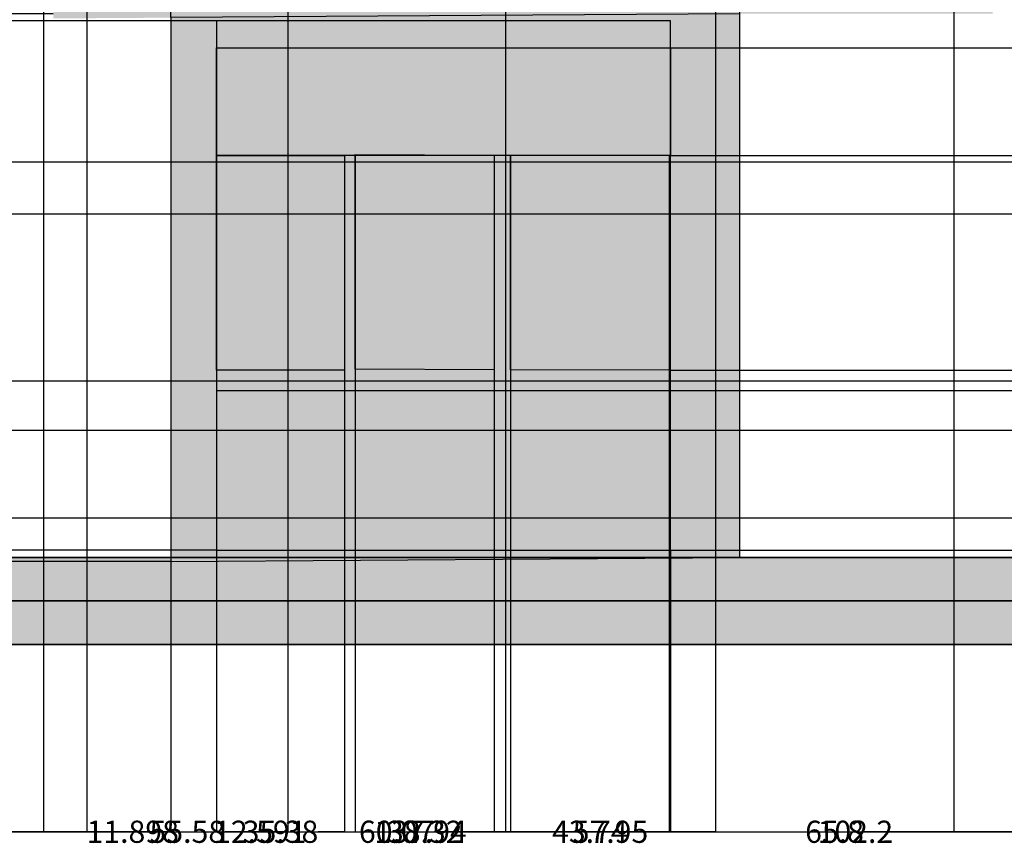
# Model space of a CAD drawing. Units: inches. Extents: x -655 to 499, y 20 to 616.
# Tile 2 of 7: x -409 to -137, y 20 to 248. Entities that reach past the tile are written whole.
import ezdxf

# ---------------------------------------------------------------- set-up
doc = ezdxf.new("R2010")
doc.units = ezdxf.units.IN
doc.header["$MEASUREMENT"] = 0
for name, color, linetype, lineweight in [('A-ANNO-DIMS', 2, 'Continuous', 18), ('A-ELEV', 7, 'Continuous', 35), ('A-ELEV-PATT', 9, 'Continuous', 13), ('A-GLAZ', 3, 'Continuous', 25), ('C-TOPO', 18, 'Continuous', 18)]:
    doc.layers.add(name, color=color, linetype=linetype, lineweight=lineweight)
doc.styles.get("Standard").update_dxf_attribs({"font": 'arial.ttf'})
doc.dimstyles.get("Standard").update_dxf_attribs({"dimtxt": 6.125, "dimasz": 0.18, "dimexe": 0.18, "dimexo": 0.0625, "dimgap": 0.09, "dimtad": 0, "dimtih": 1, "dimtoh": 1, "dimdec": 4, "dimzin": 0, "dimdsep": 46, "dimlunit": 4, "dimtxsty": 'Standard', "dimcen": 0.09, "dimadec": 0, "dimazin": 0, "dimtfac": 1, "dimtdec": 4, "dimtofl": 0, "dimtmove": 0, "dimatfit": 3, "dimfxl": 1, "dimtolj": 1, "dimtzin": 0, "dimarcsym": 0})

# ---------------------------------------------------------------- blocks, each defined once
blk = doc.blocks.new('*D10')
at = {"layer": 'A-ANNO-DIMS', "color": 0, "lineweight": -2, "transparency": 16777216}
for p, q in [((434.11, 393.11), (434.11, 23.7)), ((-590.16, 75.57), (-590.16, 23.7)), ((-589.98, 23.88), (-90.54, 23.88)), ((433.93, 23.88), (-65.51, 23.88))]:
    blk.add_line(p, q, dxfattribs=at)
at = {"layer": 'A-ANNO-DIMS', "color": 0, "transparency": 16777216}
for points in [[(-589.98, 23.91), (-589.98, 23.85), (-590.16, 23.88)], [(433.93, 23.91), (433.93, 23.85), (434.11, 23.88)]]:
    blk.add_solid(points, dxfattribs=at)
at = {"layer": 'Defpoints', "color": 0, "transparency": 16777216}
for p in [(434.11, 393.17), (-590.16, 75.63), (434.11, 23.88)]:
    blk.add_point(p, dxfattribs=at)
at = {"layer": 'A-ANNO-DIMS', "color": 0, "transparency": 16777216, "insert": (-78.02, 23.88), "char_height": 6.125, "attachment_point": 5}
blk.add_mtext('\\A1;1024.3', dxfattribs=at)
blk = doc.blocks.new('*D12')
at = {"layer": 'A-ANNO-DIMS', "color": 0, "lineweight": -2, "transparency": 16777216}
for p, q in [((-493.03, 99.57), (-493.03, 23.7)), ((-366.94, 98.47), (-366.94, 23.7)), ((-492.85, 23.88), (-439.53, 23.88)), ((-367.12, 23.88), (-420.44, 23.88))]:
    blk.add_line(p, q, dxfattribs=at)
at = {"layer": 'A-ANNO-DIMS', "color": 0, "transparency": 16777216}
for points in [[(-492.85, 23.91), (-492.85, 23.85), (-493.03, 23.88)], [(-367.12, 23.91), (-367.12, 23.85), (-366.94, 23.88)]]:
    blk.add_solid(points, dxfattribs=at)
at = {"layer": 'Defpoints', "color": 0, "transparency": 16777216}
for p in [(-493.03, 99.63), (-366.94, 98.53), (-366.94, 23.88)]:
    blk.add_point(p, dxfattribs=at)
at = {"layer": 'A-ANNO-DIMS', "color": 0, "transparency": 16777216, "insert": (-429.99, 23.88), "char_height": 6.125, "attachment_point": 5}
blk.add_mtext('\\A1;126.1', dxfattribs=at)
blk = doc.blocks.new('*D13')
at = {"layer": 'A-ANNO-DIMS', "color": 0, "lineweight": -2, "transparency": 16777216}
for p, q in [((-229.01, 101.57), (-229.01, 23.7)), ((-366.94, 98.47), (-366.94, 23.7)), ((-366.76, 23.88), (-310.48, 23.88)), ((-229.19, 23.88), (-285.47, 23.88))]:
    blk.add_line(p, q, dxfattribs=at)
at = {"layer": 'A-ANNO-DIMS', "color": 0, "transparency": 16777216}
for points in [[(-366.76, 23.91), (-366.76, 23.85), (-366.94, 23.88)], [(-229.19, 23.91), (-229.19, 23.85), (-229.01, 23.88)]]:
    blk.add_solid(points, dxfattribs=at)
at = {"layer": 'Defpoints', "color": 0, "transparency": 16777216}
for p in [(-229.01, 101.63), (-366.94, 98.53), (-229.01, 23.88)]:
    blk.add_point(p, dxfattribs=at)
at = {"layer": 'A-ANNO-DIMS', "color": 0, "transparency": 16777216, "insert": (-297.98, 23.88), "char_height": 6.125, "attachment_point": 5}
blk.add_mtext('\\A1;137.94', dxfattribs=at)
blk = doc.blocks.new('*D14')
at = {"layer": 'A-ANNO-DIMS', "color": 0, "lineweight": -2, "transparency": 16777216}
for p, q in [((-229.01, 101.57), (-229.01, 23.7)), ((-126.81, 99.57), (-126.81, 23.7)), ((-228.83, 23.88), (-188.01, 23.88)), ((-126.99, 23.88), (-167.8, 23.88))]:
    blk.add_line(p, q, dxfattribs=at)
at = {"layer": 'A-ANNO-DIMS', "color": 0, "transparency": 16777216}
for points in [[(-228.83, 23.91), (-228.83, 23.85), (-229.01, 23.88)], [(-126.99, 23.91), (-126.99, 23.85), (-126.81, 23.88)]]:
    blk.add_solid(points, dxfattribs=at)
at = {"layer": 'Defpoints', "color": 0, "transparency": 16777216}
for p in [(-229.01, 101.63), (-126.81, 99.63), (-126.81, 23.88)]:
    blk.add_point(p, dxfattribs=at)
at = {"layer": 'A-ANNO-DIMS', "color": 0, "transparency": 16777216, "insert": (-177.91, 23.88), "char_height": 6.125, "attachment_point": 5}
blk.add_mtext('\\A1;102.2', dxfattribs=at)
blk = doc.blocks.new('*D21')
at = {"layer": 'A-ANNO-DIMS', "color": 0, "lineweight": -2, "transparency": 16777216}
for p, q in [((179.11, 559.78), (486.04, 559.78)), ((485.86, 559.6), (485.86, 320.92)), ((485.86, 75.81), (485.86, 314.49)), ((-590.1, 75.63), (486.04, 75.63))]:
    blk.add_line(p, q, dxfattribs=at)
at = {"layer": 'A-ANNO-DIMS', "color": 0, "transparency": 16777216}
for points in [[(485.83, 559.6), (485.89, 559.6), (485.86, 559.78)], [(485.83, 75.81), (485.89, 75.81), (485.86, 75.63)]]:
    blk.add_solid(points, dxfattribs=at)
at = {"layer": 'Defpoints', "color": 0, "transparency": 16777216}
for p in [(179.05, 559.78), (485.86, 559.78), (-590.16, 75.63)]:
    blk.add_point(p, dxfattribs=at)
at = {"layer": 'A-ANNO-DIMS', "color": 0, "transparency": 16777216, "insert": (485.86, 317.7), "char_height": 6.125, "attachment_point": 5}
blk.add_mtext('\\A1;484.15', dxfattribs=at)
blk = doc.blocks.new('*D25')
at = {"layer": 'A-ANNO-DIMS', "color": 0, "lineweight": -2, "transparency": 16777216}
for p, q in [((-399.44, 249.84), (-642.09, 249.84)), ((-641.91, 249.66), (-641.91, 177.41)), ((-641.91, 98.71), (-641.91, 170.97)), ((-367.01, 98.53), (-642.09, 98.53))]:
    blk.add_line(p, q, dxfattribs=at)
at = {"layer": 'A-ANNO-DIMS', "color": 0, "transparency": 16777216}
for points in [[(-641.94, 249.66), (-641.88, 249.66), (-641.91, 249.84)], [(-641.94, 98.71), (-641.88, 98.71), (-641.91, 98.53)]]:
    blk.add_solid(points, dxfattribs=at)
at = {"layer": 'Defpoints', "color": 0, "transparency": 16777216}
for p in [(-399.38, 249.84), (-641.91, 98.53), (-366.94, 98.53)]:
    blk.add_point(p, dxfattribs=at)
at = {"layer": 'A-ANNO-DIMS', "color": 0, "transparency": 16777216, "insert": (-641.91, 174.19), "char_height": 6.125, "attachment_point": 5}
blk.add_mtext('\\A1;151.3', dxfattribs=at)
blk = doc.blocks.new('*D38')
at = {"layer": 'A-ANNO-DIMS', "color": 0, "lineweight": -2, "transparency": 16777216}
for p, q in [((-402.07, 316.99), (-402.07, 23.7)), ((-390.18, 316.99), (-390.18, 23.7)), ((-401.89, 23.88), (-390.36, 23.88)), ((-390.18, 23.88), (-390, 23.88))]:
    blk.add_line(p, q, dxfattribs=at)
at = {"layer": 'A-ANNO-DIMS', "color": 0, "transparency": 16777216}
for points in [[(-401.89, 23.91), (-401.89, 23.85), (-402.07, 23.88)], [(-390.36, 23.91), (-390.36, 23.85), (-390.18, 23.88)]]:
    blk.add_solid(points, dxfattribs=at)
at = {"layer": 'Defpoints', "color": 0, "transparency": 16777216}
for p in [(-402.07, 317.05), (-390.18, 317.05), (-390.18, 23.88)]:
    blk.add_point(p, dxfattribs=at)
at = {"layer": 'A-ANNO-DIMS', "color": 0, "transparency": 16777216, "insert": (-377.47, 23.88), "char_height": 6.125, "attachment_point": 5}
blk.add_mtext('\\A1;11.898', dxfattribs=at)
blk = doc.blocks.new('*D39')
at = {"layer": 'A-ANNO-DIMS', "color": 0, "lineweight": -2, "transparency": 16777216}
for p, q in [((-390.18, 316.99), (-390.18, 23.7)), ((-334.6, 316.99), (-334.6, 23.7)), ((-390, 23.88), (-372.82, 23.88)), ((-334.78, 23.88), (-351.96, 23.88))]:
    blk.add_line(p, q, dxfattribs=at)
at = {"layer": 'A-ANNO-DIMS', "color": 0, "transparency": 16777216}
for points in [[(-390, 23.91), (-390, 23.85), (-390.18, 23.88)], [(-334.78, 23.91), (-334.78, 23.85), (-334.6, 23.88)]]:
    blk.add_solid(points, dxfattribs=at)
at = {"layer": 'Defpoints', "color": 0, "transparency": 16777216}
for p in [(-390.18, 317.05), (-334.6, 317.05), (-334.6, 23.88)]:
    blk.add_point(p, dxfattribs=at)
at = {"layer": 'A-ANNO-DIMS', "color": 0, "transparency": 16777216, "insert": (-362.39, 23.88), "char_height": 6.125, "attachment_point": 5}
blk.add_mtext('\\A1;55.58', dxfattribs=at)
blk = doc.blocks.new('*D40')
at = {"layer": 'A-ANNO-DIMS', "color": 0, "lineweight": -2, "transparency": 16777216}
for p, q in [((-334.6, 316.99), (-334.6, 23.7)), ((-274.52, 316.99), (-274.52, 23.7)), ((-334.42, 23.88), (-315, 23.88)), ((-274.7, 23.88), (-294.12, 23.88))]:
    blk.add_line(p, q, dxfattribs=at)
at = {"layer": 'A-ANNO-DIMS', "color": 0, "transparency": 16777216}
for points in [[(-334.42, 23.91), (-334.42, 23.85), (-334.6, 23.88)], [(-274.7, 23.91), (-274.7, 23.85), (-274.52, 23.88)]]:
    blk.add_solid(points, dxfattribs=at)
at = {"layer": 'Defpoints', "color": 0, "transparency": 16777216}
for p in [(-334.6, 317.05), (-274.52, 317.05), (-274.52, 23.88)]:
    blk.add_point(p, dxfattribs=at)
at = {"layer": 'A-ANNO-DIMS', "color": 0, "transparency": 16777216, "insert": (-304.56, 23.88), "char_height": 6.125, "attachment_point": 5}
blk.add_mtext('\\A1;60.07', dxfattribs=at)
blk = doc.blocks.new('*D41')
at = {"layer": 'A-ANNO-DIMS', "color": 0, "lineweight": -2, "transparency": 16777216}
for p, q in [((-274.52, 316.99), (-274.52, 23.7)), ((-216.57, 316.99), (-216.57, 23.7)), ((-274.34, 23.88), (-256, 23.88)), ((-216.75, 23.88), (-235.1, 23.88))]:
    blk.add_line(p, q, dxfattribs=at)
at = {"layer": 'A-ANNO-DIMS', "color": 0, "transparency": 16777216}
for points in [[(-274.34, 23.91), (-274.34, 23.85), (-274.52, 23.88)], [(-216.75, 23.91), (-216.75, 23.85), (-216.57, 23.88)]]:
    blk.add_solid(points, dxfattribs=at)
at = {"layer": 'Defpoints', "color": 0, "transparency": 16777216}
for p in [(-274.52, 317.05), (-216.57, 317.05), (-216.57, 23.88)]:
    blk.add_point(p, dxfattribs=at)
at = {"layer": 'A-ANNO-DIMS', "color": 0, "transparency": 16777216, "insert": (-245.55, 23.88), "char_height": 6.125, "attachment_point": 5}
blk.add_mtext('\\A1;57.95', dxfattribs=at)
blk = doc.blocks.new('*D42')
at = {"layer": 'A-ANNO-DIMS', "color": 0, "lineweight": -2, "transparency": 16777216}
for p, q in [((-216.57, 316.99), (-216.57, 23.7)), ((-150.77, 316.99), (-150.77, 23.7)), ((-216.39, 23.88), (-191.74, 23.88)), ((-150.95, 23.88), (-175.6, 23.88))]:
    blk.add_line(p, q, dxfattribs=at)
at = {"layer": 'A-ANNO-DIMS', "color": 0, "transparency": 16777216}
for points in [[(-216.39, 23.91), (-216.39, 23.85), (-216.57, 23.88)], [(-150.95, 23.91), (-150.95, 23.85), (-150.77, 23.88)]]:
    blk.add_solid(points, dxfattribs=at)
at = {"layer": 'Defpoints', "color": 0, "transparency": 16777216}
for p in [(-216.57, 317.05), (-150.77, 317.05), (-150.77, 23.88)]:
    blk.add_point(p, dxfattribs=at)
at = {"layer": 'A-ANNO-DIMS', "color": 0, "transparency": 16777216, "insert": (-183.67, 23.88), "char_height": 6.125, "attachment_point": 5}
blk.add_mtext('\\A1;65.8', dxfattribs=at)
blk = doc.blocks.new('*D43')
at = {"layer": 'A-ANNO-DIMS', "color": 0, "lineweight": -2, "transparency": 16777216}
for p, q in [((-366.94, 248.81), (-366.94, 611.71)), ((-366.76, 611.53), (-300.88, 611.53)), ((-209.98, 611.53), (-275.87, 611.53)), ((-209.8, 99.69), (-209.8, 611.71))]:
    blk.add_line(p, q, dxfattribs=at)
at = {"layer": 'A-ANNO-DIMS', "color": 0, "transparency": 16777216}
for points in [[(-366.76, 611.56), (-366.76, 611.5), (-366.94, 611.53)], [(-209.98, 611.56), (-209.98, 611.5), (-209.8, 611.53)]]:
    blk.add_solid(points, dxfattribs=at)
at = {"layer": 'Defpoints', "color": 0, "transparency": 16777216}
for p in [(-209.8, 611.53), (-366.94, 248.74), (-209.8, 99.63)]:
    blk.add_point(p, dxfattribs=at)
at = {"layer": 'A-ANNO-DIMS', "color": 0, "transparency": 16777216, "insert": (-288.37, 611.53), "char_height": 6.125, "attachment_point": 5}
blk.add_mtext('\\A1;157.14', dxfattribs=at)
blk = doc.blocks.new('*D44')
at = {"layer": 'A-ANNO-DIMS', "color": 0, "lineweight": -2, "transparency": 16777216}
for p, q in [((-366.94, 248.68), (-366.94, 23.7)), ((-354.35, 247.78), (-354.35, 23.7)), ((-366.76, 23.88), (-354.53, 23.88)), ((-354.35, 23.88), (-354.17, 23.88))]:
    blk.add_line(p, q, dxfattribs=at)
at = {"layer": 'A-ANNO-DIMS', "color": 0, "transparency": 16777216}
for points in [[(-366.76, 23.91), (-366.76, 23.85), (-366.94, 23.88)], [(-354.53, 23.91), (-354.53, 23.85), (-354.35, 23.88)]]:
    blk.add_solid(points, dxfattribs=at)
at = {"layer": 'Defpoints', "color": 0, "transparency": 16777216}
for p in [(-366.94, 248.74), (-354.35, 247.84), (-354.35, 23.88)]:
    blk.add_point(p, dxfattribs=at)
at = {"layer": 'A-ANNO-DIMS', "color": 0, "transparency": 16777216, "insert": (-342.25, 23.88), "char_height": 6.125, "attachment_point": 5}
blk.add_mtext('\\A1;12.591', dxfattribs=at)
blk = doc.blocks.new('*D45')
at = {"layer": 'A-ANNO-DIMS', "color": 0, "lineweight": -2, "transparency": 16777216}
for p, q in [((-354.35, 210.58), (-354.35, 23.7)), ((-318.97, 210.58), (-318.97, 23.7)), ((-354.17, 23.88), (-347.09, 23.88)), ((-319.15, 23.88), (-326.24, 23.88))]:
    blk.add_line(p, q, dxfattribs=at)
at = {"layer": 'A-ANNO-DIMS', "color": 0, "transparency": 16777216}
for points in [[(-354.17, 23.91), (-354.17, 23.85), (-354.35, 23.88)], [(-319.15, 23.91), (-319.15, 23.85), (-318.97, 23.88)]]:
    blk.add_solid(points, dxfattribs=at)
at = {"layer": 'Defpoints', "color": 0, "transparency": 16777216}
for p in [(-354.35, 210.64), (-318.97, 210.64), (-318.97, 23.88)]:
    blk.add_point(p, dxfattribs=at)
at = {"layer": 'A-ANNO-DIMS', "color": 0, "transparency": 16777216, "insert": (-336.66, 23.88), "char_height": 6.125, "attachment_point": 5}
blk.add_mtext('\\A1;35.38', dxfattribs=at)
blk = doc.blocks.new('*D46')
at = {"layer": 'A-ANNO-DIMS', "color": 0, "lineweight": -2, "transparency": 16777216}
for p, q in [((-316, 210.87), (-316, 23.7)), ((-277.68, 210.74), (-277.68, 23.7)), ((-315.82, 23.88), (-307.23, 23.88)), ((-277.86, 23.88), (-286.45, 23.88))]:
    blk.add_line(p, q, dxfattribs=at)
at = {"layer": 'A-ANNO-DIMS', "color": 0, "transparency": 16777216}
for points in [[(-315.82, 23.91), (-315.82, 23.85), (-316, 23.88)], [(-277.86, 23.91), (-277.86, 23.85), (-277.68, 23.88)]]:
    blk.add_solid(points, dxfattribs=at)
at = {"layer": 'Defpoints', "color": 0, "transparency": 16777216}
for p in [(-316, 210.93), (-277.68, 210.8), (-277.68, 23.88)]:
    blk.add_point(p, dxfattribs=at)
at = {"layer": 'A-ANNO-DIMS', "color": 0, "transparency": 16777216, "insert": (-296.84, 23.88), "char_height": 6.125, "attachment_point": 5}
blk.add_mtext('\\A1;38.32', dxfattribs=at)
blk = doc.blocks.new('*D47')
at = {"layer": 'A-ANNO-DIMS', "color": 0, "lineweight": -2, "transparency": 16777216}
for p, q in [((-273.11, 210.74), (-273.11, 23.7)), ((-229.36, 210.58), (-229.36, 23.7)), ((-272.93, 23.88), (-261.77, 23.88)), ((-229.54, 23.88), (-240.7, 23.88))]:
    blk.add_line(p, q, dxfattribs=at)
at = {"layer": 'A-ANNO-DIMS', "color": 0, "transparency": 16777216}
for points in [[(-272.93, 23.91), (-272.93, 23.85), (-273.11, 23.88)], [(-229.54, 23.91), (-229.54, 23.85), (-229.36, 23.88)]]:
    blk.add_solid(points, dxfattribs=at)
at = {"layer": 'Defpoints', "color": 0, "transparency": 16777216}
for p in [(-273.11, 210.8), (-229.36, 210.64), (-229.36, 23.88)]:
    blk.add_point(p, dxfattribs=at)
at = {"layer": 'A-ANNO-DIMS', "color": 0, "transparency": 16777216, "insert": (-251.23, 23.88), "char_height": 6.125, "attachment_point": 5}
blk.add_mtext('\\A1;43.74', dxfattribs=at)
blk = doc.blocks.new('*D48')
at = {"layer": 'A-ANNO-DIMS', "color": 0, "lineweight": -2, "transparency": 16777216}
for p, q in [((-228.95, 145.8), (486.04, 145.8)), ((485.86, 145.62), (485.86, 126.88)), ((485.86, 101.81), (485.86, 120.55)), ((-228.95, 101.63), (486.04, 101.63))]:
    blk.add_line(p, q, dxfattribs=at)
at = {"layer": 'A-ANNO-DIMS', "color": 0, "transparency": 16777216}
for points in [[(485.83, 145.62), (485.89, 145.62), (485.86, 145.8)], [(485.83, 101.81), (485.89, 101.81), (485.86, 101.63)]]:
    blk.add_solid(points, dxfattribs=at)
at = {"layer": 'Defpoints', "color": 0, "transparency": 16777216}
for p in [(-229.01, 145.8), (485.86, 145.8), (-229.01, 101.63)]:
    blk.add_point(p, dxfattribs=at)
at = {"layer": 'A-ANNO-DIMS', "color": 0, "transparency": 16777216, "insert": (485.86, 123.72), "char_height": 6.125, "attachment_point": 5}
blk.add_mtext('\\A1;44.17', dxfattribs=at)
blk = doc.blocks.new('*D49')
at = {"layer": 'A-ANNO-DIMS', "color": 0, "lineweight": -2, "transparency": 16777216}
for p, q in [((-229.3, 210.64), (486.04, 210.64)), ((485.86, 210.46), (485.86, 184.21)), ((485.86, 151.52), (485.86, 177.77)), ((-229.3, 151.34), (486.04, 151.34))]:
    blk.add_line(p, q, dxfattribs=at)
at = {"layer": 'A-ANNO-DIMS', "color": 0, "transparency": 16777216}
for points in [[(485.83, 210.46), (485.89, 210.46), (485.86, 210.64)], [(485.83, 151.52), (485.89, 151.52), (485.86, 151.34)]]:
    blk.add_solid(points, dxfattribs=at)
at = {"layer": 'Defpoints', "color": 0, "transparency": 16777216}
for p in [(-229.36, 210.64), (485.86, 210.64), (-229.36, 151.34)]:
    blk.add_point(p, dxfattribs=at)
at = {"layer": 'A-ANNO-DIMS', "color": 0, "transparency": 16777216, "insert": (485.86, 180.99), "char_height": 6.125, "attachment_point": 5}
blk.add_mtext('\\A1;59.3', dxfattribs=at)
blk = doc.blocks.new('*D50')
at = {"layer": 'A-ANNO-DIMS', "color": 0, "lineweight": -2, "transparency": 16777216}
for p, q in [((-354.42, 247.84), (-642.09, 247.84)), ((-641.91, 247.66), (-641.91, 177.95)), ((-641.91, 101.81), (-641.91, 171.52)), ((-354.42, 101.63), (-642.09, 101.63))]:
    blk.add_line(p, q, dxfattribs=at)
at = {"layer": 'A-ANNO-DIMS', "color": 0, "transparency": 16777216}
for points in [[(-641.94, 247.66), (-641.88, 247.66), (-641.91, 247.84)], [(-641.94, 101.81), (-641.88, 101.81), (-641.91, 101.63)]]:
    blk.add_solid(points, dxfattribs=at)
at = {"layer": 'Defpoints', "color": 0, "transparency": 16777216}
for p in [(-641.91, 247.84), (-354.35, 247.84), (-354.35, 101.63)]:
    blk.add_point(p, dxfattribs=at)
at = {"layer": 'A-ANNO-DIMS', "color": 0, "transparency": 16777216, "insert": (-641.91, 174.74), "char_height": 6.125, "attachment_point": 5}
blk.add_mtext('\\A1;146.2', dxfattribs=at)
blk = doc.blocks.new('*D51')
at = {"layer": 'A-ANNO-DIMS', "color": 0, "lineweight": -2, "transparency": 16777216}
for p, q in [((-228.95, 240.42), (486.04, 240.42)), ((485.86, 240.24), (485.86, 228.75)), ((485.86, 210.82), (485.86, 222.31)), ((-228.88, 210.64), (486.04, 210.64))]:
    blk.add_line(p, q, dxfattribs=at)
at = {"layer": 'A-ANNO-DIMS', "color": 0, "transparency": 16777216}
for points in [[(485.83, 240.24), (485.89, 240.24), (485.86, 240.42)], [(485.83, 210.82), (485.89, 210.82), (485.86, 210.64)]]:
    blk.add_solid(points, dxfattribs=at)
at = {"layer": 'Defpoints', "color": 0, "transparency": 16777216}
for p in [(-229.01, 240.42), (485.86, 240.42), (-228.94, 210.64)]:
    blk.add_point(p, dxfattribs=at)
at = {"layer": 'A-ANNO-DIMS', "color": 0, "transparency": 16777216, "insert": (485.86, 225.53), "char_height": 6.125, "attachment_point": 5}
blk.add_mtext('\\A1;29.776', dxfattribs=at)
blk = doc.blocks.new('*D67')
at = {"layer": 'A-ANNO-DIMS', "color": 0, "lineweight": -2, "transparency": 16777216}
for p, q in [((-42.36, 110.53), (-642.09, 110.53)), ((-641.91, 110.35), (-641.91, 108.29)), ((-641.91, 99.81), (-641.91, 101.86)), ((-64.18, 99.63), (-642.09, 99.63))]:
    blk.add_line(p, q, dxfattribs=at)
at = {"layer": 'A-ANNO-DIMS', "color": 0, "transparency": 16777216}
for points in [[(-641.94, 110.35), (-641.88, 110.35), (-641.91, 110.53)], [(-641.94, 99.81), (-641.88, 99.81), (-641.91, 99.63)]]:
    blk.add_solid(points, dxfattribs=at)
at = {"layer": 'Defpoints', "color": 0, "transparency": 16777216}
for p in [(-42.3, 110.53), (-641.91, 99.63), (-64.12, 99.63)]:
    blk.add_point(p, dxfattribs=at)
at = {"layer": 'A-ANNO-DIMS', "color": 0, "transparency": 16777216, "insert": (-641.91, 105.08), "char_height": 6.125, "attachment_point": 5}
blk.add_mtext('\\A1;10.896', dxfattribs=at)
blk = doc.blocks.new('*D68')
at = {"layer": 'A-ANNO-DIMS', "color": 0, "lineweight": -2, "transparency": 16777216}
for p, q in [((-42.36, 134.67), (-642.09, 134.67)), ((-641.91, 134.49), (-641.91, 125.76)), ((-641.91, 110.71), (-641.91, 119.43)), ((-42.36, 110.53), (-642.09, 110.53))]:
    blk.add_line(p, q, dxfattribs=at)
at = {"layer": 'A-ANNO-DIMS', "color": 0, "transparency": 16777216}
for points in [[(-641.94, 134.49), (-641.88, 134.49), (-641.91, 134.67)], [(-641.94, 110.71), (-641.88, 110.71), (-641.91, 110.53)]]:
    blk.add_solid(points, dxfattribs=at)
at = {"layer": 'Defpoints', "color": 0, "transparency": 16777216}
for p in [(-641.91, 134.67), (-42.3, 134.67), (-42.3, 110.53)]:
    blk.add_point(p, dxfattribs=at)
at = {"layer": 'A-ANNO-DIMS', "color": 0, "transparency": 16777216, "insert": (-641.91, 122.6), "char_height": 6.125, "attachment_point": 5}
blk.add_mtext('\\A1;24.14', dxfattribs=at)
blk = doc.blocks.new('*D69')
at = {"layer": 'A-ANNO-DIMS', "color": 0, "lineweight": -2, "transparency": 16777216}
for p, q in [((-42.36, 148.31), (-642.09, 148.31)), ((-641.91, 148.13), (-641.91, 144.71)), ((-641.91, 134.85), (-641.91, 138.27)), ((-42.36, 134.67), (-642.09, 134.67))]:
    blk.add_line(p, q, dxfattribs=at)
at = {"layer": 'A-ANNO-DIMS', "color": 0, "transparency": 16777216}
for points in [[(-641.94, 148.13), (-641.88, 148.13), (-641.91, 148.31)], [(-641.94, 134.85), (-641.88, 134.85), (-641.91, 134.67)]]:
    blk.add_solid(points, dxfattribs=at)
at = {"layer": 'Defpoints', "color": 0, "transparency": 16777216}
for p in [(-641.91, 148.31), (-42.3, 148.31), (-42.3, 134.67)]:
    blk.add_point(p, dxfattribs=at)
at = {"layer": 'A-ANNO-DIMS', "color": 0, "transparency": 16777216, "insert": (-641.91, 141.49), "char_height": 6.125, "attachment_point": 5}
blk.add_mtext('\\A1;13.64', dxfattribs=at)
blk = doc.blocks.new('*D70')
at = {"layer": 'A-ANNO-DIMS', "color": 0, "lineweight": -2, "transparency": 16777216}
for p, q in [((-42.36, 194.47), (-642.09, 194.47)), ((-641.91, 194.29), (-641.91, 174.61)), ((-641.91, 148.49), (-641.91, 168.17)), ((-42.36, 148.31), (-642.09, 148.31))]:
    blk.add_line(p, q, dxfattribs=at)
at = {"layer": 'A-ANNO-DIMS', "color": 0, "transparency": 16777216}
for points in [[(-641.94, 194.29), (-641.88, 194.29), (-641.91, 194.47)], [(-641.94, 148.49), (-641.88, 148.49), (-641.91, 148.31)]]:
    blk.add_solid(points, dxfattribs=at)
at = {"layer": 'Defpoints', "color": 0, "transparency": 16777216}
for p in [(-641.91, 194.47), (-42.3, 194.47), (-42.3, 148.31)]:
    blk.add_point(p, dxfattribs=at)
at = {"layer": 'A-ANNO-DIMS', "color": 0, "transparency": 16777216, "insert": (-641.91, 171.39), "char_height": 6.125, "attachment_point": 5}
blk.add_mtext('\\A1;46.16', dxfattribs=at)
blk = doc.blocks.new('*D71')
at = {"layer": 'A-ANNO-DIMS', "color": 0, "lineweight": -2, "transparency": 16777216}
for p, q in [((-64.18, 208.79), (-642.09, 208.79)), ((-641.91, 208.61), (-641.91, 204.85)), ((-641.91, 194.65), (-641.91, 198.41)), ((-42.36, 194.47), (-642.09, 194.47))]:
    blk.add_line(p, q, dxfattribs=at)
at = {"layer": 'A-ANNO-DIMS', "color": 0, "transparency": 16777216}
for points in [[(-641.94, 208.61), (-641.88, 208.61), (-641.91, 208.79)], [(-641.94, 194.65), (-641.88, 194.65), (-641.91, 194.47)]]:
    blk.add_solid(points, dxfattribs=at)
at = {"layer": 'Defpoints', "color": 0, "transparency": 16777216}
for p in [(-641.91, 208.79), (-64.12, 208.79), (-42.3, 194.47)]:
    blk.add_point(p, dxfattribs=at)
at = {"layer": 'A-ANNO-DIMS', "color": 0, "transparency": 16777216, "insert": (-641.91, 201.63), "char_height": 6.125, "attachment_point": 5}
blk.add_mtext('\\A1;14.32', dxfattribs=at)

msp = doc.modelspace()

# ---------------------------------------------------------------- hatches: boundary and pattern name
at = {"layer": 'A-ELEV-PATT'}
h = msp.add_hatch(color=256, dxfattribs=at)
h.dxf.hatch_style = 1
h.paths.add_polyline_path([(-140.0489, 272.2618), (-399.3758, 272.2618), (-399.3758, 249.8418), (-399.3758, 248.5179), (-366.9446, 248.7444), (-209.8047, 249.8418), (-183.5755, 249.8418), (-140.0489, 249.8418)])
h.paths.add_polyline_path([(-211.7589, 317.0515), (-216.5713, 317.0515), (-216.5713, 272.2618), (-211.7589, 272.2618)])
h.paths.add_polyline_path([(-145.96, 317.0515), (-150.7725, 317.0515), (-150.7725, 272.2618), (-145.96, 272.2618)])
h.paths.add_polyline_path([(-140.5198, 321.4867), (-402.0739, 321.4867), (-402.0739, 317.0515), (-390.1757, 317.0515), (-385.3633, 317.0515), (-150.7725, 317.0515), (-145.96, 317.0515), (-140.5198, 317.0515)])
h.paths.add_polyline_path([(-269.7123, 317.0515), (-274.5248, 317.0515), (-274.5248, 272.2618), (-269.7123, 272.2618)])
h.paths.add_polyline_path([(-329.7837, 317.0515), (-334.5961, 317.0515), (-334.5961, 280.9678), (-329.7837, 280.9678)])
h.paths.add_polyline_path([(-329.7837, 280.9678), (-334.5961, 280.9678), (-334.5961, 272.2618), (-329.7837, 272.2618)])
h.paths.add_polyline_path([(-385.3633, 317.0515), (-390.1757, 317.0515), (-390.1757, 272.2618), (-385.3633, 272.2618)])
h.paths.add_polyline_path([(-229.0087, 240.4184), (-354.3532, 240.4184), (-354.2854, 210.6425), (-315.9956, 210.6425), (-315.9956, 210.9348), (-277.6793, 210.7995), (-277.6793, 210.6425), (-273.1052, 210.6425), (-273.1052, 210.7995), (-229.3637, 210.6425), (-229.0087, 210.6425)])
h.paths.add_polyline_path([(-229.0087, 145.8007), (-354.3532, 145.8007), (-354.3532, 101.6296), (-229.0087, 101.6296)])
h.paths.add_polyline_path([(-229.0087, 210.6425), (-229.3637, 210.6425), (-229.3637, 151.3385), (-273.1052, 151.4955), (-273.1052, 210.6425), (-277.6793, 210.6425), (-277.6793, 151.4955), (-315.9956, 151.6308), (-315.9956, 210.6425), (-318.9742, 210.6425), (-318.9742, 151.3385), (-354.3532, 151.3385), (-354.3532, 145.8007), (-229.0087, 145.8007)])
h.paths.add_polyline_path([(-229.0087, 247.8418), (-354.3532, 247.8418), (-354.3532, 240.4184), (-229.0087, 240.4184)])
h.paths.add_polyline_path([(4.4271, 93.6296), (-100.4134, 93.6296), (-124.8077, 93.6296), (-126.8077, 93.6296), (-126.8077, 87.6296), (4.4271, 87.6296)])
h.paths.add_polyline_path([(4.4271, 99.6296), (-100.4134, 99.6296), (-100.4134, 93.6296), (4.4271, 93.6296)])
h.paths.add_polyline_path([(99.4982, 99.6296), (6.4271, 99.6296), (6.4271, 93.6296), (99.4982, 93.6296)])
h.paths.add_polyline_path([(99.4982, 93.6296), (6.4271, 93.6296), (6.4271, 87.6296), (99.4982, 87.6296)])
h.paths.add_polyline_path([(304.2843, 311.436), (230.0144, 311.076), (230.0144, 282.9577), (270.6361, 282.9577), (304.4665, 273.8535)])
h.paths.add_polyline_path([(304.1054, 348.3371), (304.1054, 356.2861), (230.0144, 356.2861), (230.0144, 348.3443), (230.0144, 311.076), (304.2843, 311.436)])
h.paths.add_polyline_path([(255.5586, 316.5111), (255.5586, 350.0185), (275.6848, 350.0185), (275.6848, 316.5111)], flags=16)
h.paths.add_polyline_path([(278.0676, 316.5111), (278.0676, 350.0185), (301.4074, 350.0185), (301.4074, 316.5111)], flags=16)
h.paths.add_polyline_path([(253.2029, 316.5111), (233.8107, 316.5111), (233.8107, 350.0185), (253.2029, 350.0185)], flags=16)
h.paths.add_polyline_path([(179.0482, 559.7795), (153.2347, 535.8185), (165.0976, 535.8185), (192.9989, 535.8185), (201.2897, 535.8185)])
h.paths.add_polyline_path([(347.8163, 516.7932), (322.0028, 492.8322), (333.8657, 492.8322), (361.7669, 492.8322), (370.0577, 492.8322)])
h = msp.add_hatch(color=256, dxfattribs=at)
h.dxf.hatch_style = 1
h.paths.add_polyline_path([(-209.8047, 249.8418), (-366.9446, 248.7444), (-366.9446, 98.5321), (-209.8047, 99.6296)])
h.paths.add_polyline_path([(-229.0087, 101.6296), (-354.3532, 101.6296), (-354.3532, 247.8418), (-229.0087, 247.8418), (-229.0087, 240.4184), (-228.941, 210.6425), (-229.0087, 210.6425)], flags=16)
h.paths.add_polyline_path([(-229.3637, 151.3385), (-273.1052, 151.4955), (-273.1052, 210.7995), (-229.3637, 210.6425)], flags=0)
h.paths.add_polyline_path([(-277.6793, 151.4955), (-315.9956, 151.6308), (-315.9956, 210.9348), (-277.6793, 210.7995)], flags=0)
h.paths.add_polyline_path([(-318.9742, 151.3385), (-354.3532, 151.3385), (-354.3532, 210.6425), (-318.9742, 210.6425)], flags=0)
h.paths.add_polyline_path([(230.0144, 348.3443), (230.0144, 356.2861), (304.1054, 356.2861), (304.1054, 348.3371), (304.4665, 273.8535), (307.4704, 273.0451), (307.1054, 348.3443), (307.1054, 359.2861), (227.0144, 359.2861), (227.0144, 348.3443), (227.0144, 282.9577), (230.0144, 282.9577)])
h = msp.add_hatch(color=256, dxfattribs=at)
h.dxf.hatch_style = 1
h.paths.add_polyline_path([(-329.7837, 350.1333), (-347.0336, 350.1333), (-347.0336, 321.4867), (-329.7837, 321.4867)])
h.paths.add_polyline_path([(-294.1413, 350.1333), (-311.3912, 350.1333), (-311.3912, 321.4867), (-294.1413, 321.4867)])
h.paths.add_polyline_path([(-294.1413, 317.0515), (-311.3912, 317.0515), (-311.3912, 280.9678), (-294.1413, 280.9678)])
h.paths.add_polyline_path([(-334.5961, 317.0515), (-347.0336, 317.0515), (-347.0336, 280.9678), (-334.5961, 280.9678)])
h.paths.add_polyline_path([(-244.6859, 336.719), (-258.4486, 336.719), (-258.4486, 347.0139), (-244.6859, 347.0139), (-244.6859, 350.1333), (-261.9358, 350.1333), (-261.9358, 321.4867), (-244.6859, 321.4867)])
h.paths.add_polyline_path([(-244.6859, 317.0515), (-261.9358, 317.0515), (-261.9358, 280.9678), (-244.6859, 280.9678)])
h.paths.add_polyline_path([(-244.6859, 347.0139), (-258.4486, 347.0139), (-258.4486, 336.719), (-244.6859, 336.719)], flags=17)
h.paths.add_polyline_path([(-318.9742, 210.6425), (-354.3532, 210.6425), (-354.3532, 151.3385), (-318.9742, 151.3385)])
h.paths.add_polyline_path([(-277.6793, 210.6425), (-315.9956, 210.6425), (-315.9956, 151.6308), (-277.6793, 151.4955)])
h.paths.add_polyline_path([(-229.3637, 210.6425), (-273.1052, 210.6425), (-273.1052, 151.4955), (-229.3637, 151.3385)])
h.paths.add_polyline_path([(-19.537, 192.4712), (-40.2951, 192.4712), (-40.2951, 150.3082), (-19.537, 150.3082)])
h.paths.add_polyline_path([(2.4271, 231.274), (-62.1158, 231.274), (-62.1158, 210.7923), (2.4271, 210.7923)])
h.paths.add_polyline_path([(72.97, 231.274), (8.4271, 231.274), (8.4271, 210.7923), (72.97, 210.7923)])
h.paths.add_polyline_path([(51.0059, 192.4712), (30.2478, 192.4712), (30.2478, 150.3082), (51.0059, 150.3082)])
h.paths.add_polyline_path([(51.0059, 132.6671), (30.2478, 132.6671), (30.2478, 112.5254), (51.0059, 112.5254)])
h.paths.add_polyline_path([(-19.537, 132.6671), (-40.2951, 132.6671), (-40.2951, 112.5254), (-19.537, 112.5254)])
h.paths.add_polyline_path([(275.6848, 350.0185), (255.5586, 350.0185), (255.5586, 316.5111), (275.6848, 316.5111)])
h.paths.add_polyline_path([(301.4074, 350.0185), (278.0676, 350.0185), (278.0676, 316.5111), (301.4074, 316.5111)])
h.paths.add_polyline_path([(253.2029, 350.0185), (233.8107, 350.0185), (233.8107, 316.5111), (253.2029, 316.5111)])
h = msp.add_hatch(color=256, dxfattribs=at)
h.dxf.hatch_style = 1
h.paths.add_polyline_path([(-126.8077, 93.6296), (-126.8077, 99.6296), (-145.6102, 99.6296), (-209.8047, 99.6296), (-366.9446, 98.5321), (-366.9446, 99.6296), (-506.835, 99.6296), (-573.6788, 99.6296), (-573.6788, 87.6296), (-506.835, 87.6296), (-161.7817, 87.6296), (-126.8077, 87.6296)])
h.paths.add_polyline_path([(419.8436, 99.6296), (99.4982, 99.6296), (99.4982, 87.6296), (419.8436, 87.6296)])
h.paths.add_polyline_path([(-100.4134, 99.6296), (-124.8077, 99.6296), (-124.8077, 93.6296), (-100.4134, 93.6296)])
h.paths.add_polyline_path([(-124.8077, 243.6296), (-126.8077, 243.6296), (-126.8077, 99.6296), (-124.8077, 99.6296)])
h.paths.add_polyline_path([(-124.8077, 99.6296), (-126.8077, 99.6296), (-126.8077, 93.6296), (-124.8077, 93.6296)])
at = {"layer": 'C-TOPO'}
h = msp.add_hatch(dxfattribs=at)
h.set_pattern_fill('GRAVEL', color=256, scale=2.2)
h.set_pattern_definition([(228.012788, (1.584, 2.2), (-17.6, -19.8), [0.295979, -29.301994]), (184.96974, (1.386, 1.98), (26.4, 2.2), [0.5079096, -50.2830345]), (132.510447, (0.88, 1.936), (22, -24.2), [0.3581336, -35.455272]), (267.27369, (0.022, 1.386), (2.2, 44), [0.4625236, -45.789828]), (292.833654, (0, 0.924), (-11, 26.4), [0.453541, -44.900621]), (357.27369, (0.176, 0.506), (-44, 2.2), [0.4625236, -45.789828]), (37.69424, (0.638, 0.484), (-28.6, -22), [0.611664, -60.554667]), (72.255328, (1.122, 0.858), (15.4, 48.4), [0.5774736, -57.169907]), (121.429566, (1.298, 1.408), (-17.6, 28.6), [0.46409, -45.944961]), (175.23636, (1.056, 1.804), (24.2, -2.2), [0.5298304, -25.961678]), (222.397438, (0.528, 1.848), (-26.4, -24.2), [0.6851856, -67.833425]), (138.814075, (2.2, 1.364), (-15.4, 13.2), [0.233862, -23.1524586]), (171.469234, (2.024, 1.518), (28.6, -4.4), [0.4449214, -44.047325]), (225, (1.584, 1.584), (-2e-16, -2.2), [0.311126, -2.800144]), (203.19859, (1.43, 1.848), (11, 4.4), [0.1675476, -16.587153]), (291.80141, (1.276, 1.782), (-2.2, 6.6), [0.2369466, -11.610416]), (30.96376, (1.364, 1.562), (6.6, 4.4), [0.384844, -12.44325]), (161.56505, (1.694, 1.76), (4.4, -2.2), [0.27828, -6.678731]), (16.38954, (0, 1.782), (22, 6.6), [0.38984, -38.594259]), (70.346176, (0.374, 1.892), (-8.8, -24.2), [0.327054, -32.378297]), (293.19859, (1.694, 2.2), (-4.4, 11), [0.335093, -16.419608]), (343.61046, (1.826, 1.892), (-22, 6.6), [0.38984, -38.594259]), (339.443955, (0, 0.418), (-11, 4.4), [0.375936, -18.420872]), (294.77514, (0.352, 0.286), (-11, 24.2), [0.3149916, -31.184215]), (66.80141, (1.716, 0), (4.4, 11), [0.335093, -16.419608]), (17.354025, (1.848, 0.308), (-28.6, -8.8), [0.368788, -36.509932]), (69.443955, (0.638, 0), (-4.4, -11), [0.187968, -18.60884]), (101.30993, (1.584, 0), (-2.2, 8.8), [0.112178, -11.105665]), (165.96376, (1.562, 0.11), (6.6, -2.2), [0.453541, -8.617291]), (186.009006, (1.122, 0.22), (22, 2.2), [0.42031, -41.610631]), (303.69007, (1.364, 1.364), (-2.2, 4.4), [0.3172884, -7.6149244]), (353.157227, (1.54, 1.1), (37.4, -4.4), [0.553947, -54.840638]), (60.945396, (2.09, 1.034), (-8.8, -15.4), [0.226503, -22.423883]), (90, (2.2, 1.232), (-2.2, 2.2), [0.132, -2.068]), (120.256437, (1.078, 0.286), (8.8, -15.4), [0.305633, -30.257744]), (48.012788, (0.924, 0.55), (17.6, 19.8), [0.5919584, -29.0060145]), (0, (1.32, 0.99), (2.2, 2.2), [0.572, -1.628]), (325.304846, (1.892, 0.99), (22, -15.4), [0.347851, -34.4372035]), (254.054604, (2.178, 0.792), (-2.2, -8.8), [0.3203244, -15.695917]), (207.645975, (2.09, 0.484), (-41.8, -22), [0.521543, -51.632843]), (175.426079, (1.628, 0.242), (-28.6, 2.2), [0.551758, -54.6239615])])
h.paths.add_polyline_path([(419.8436, 87.6296), (99.4982, 87.6296), (-161.7817, 87.6296), (-506.835, 87.6296), (-573.6788, 87.6296), (-590.1625, 87.6296), (-590.1625, 75.6296), (-496.5301, 75.6296), (-76.7836, 75.6296), (99.4982, 75.6296), (419.8436, 75.6296)])

# ---------------------------------------------------------------- linework, layer by layer
at = {"layer": 'A-ELEV'}
for p, q in [((-145.6102, 99.6296), (-506.835, 99.6296)), ((99.4982, 99.6296), (-145.6102, 99.6296)), ((-161.7817, 87.6296), (-506.835, 87.6296)), ((99.4982, 87.6296), (-161.7817, 87.6296)), ((-76.7836, 75.6296), (-496.5301, 75.6296))]:
    msp.add_line(p, q, dxfattribs=at)
at = {"layer": 'A-GLAZ'}
msp.add_line((-354.3532, 145.8007), (-229.0087, 145.8007), dxfattribs=at)
for points in [[(-366.9446, 98.5321), (-209.8047, 99.6296), (-209.8047, 249.8418), (-366.9446, 248.7444)], [(-354.3532, 101.6296), (-229.0087, 101.6296), (-229.0087, 247.8418), (-354.3532, 247.8418)], [(-354.3532, 240.4184), (-229.0087, 240.4184), (-228.941, 210.6425), (-354.2854, 210.6425)], [(-354.3532, 210.6425), (-318.9742, 210.6425), (-318.9742, 151.3385), (-354.3532, 151.3385)], [(-315.9956, 210.9348), (-277.6793, 210.7995), (-277.6793, 151.4955), (-315.9956, 151.6308)], [(-273.1052, 210.7995), (-229.3637, 210.6425), (-229.3637, 151.3385), (-273.1052, 151.4955)]]:
    msp.add_lwpolyline(points, close=True, dxfattribs=at)

# ---------------------------------------------------------------- dimensions: what is measured, and where the dimension line sits
at = {"layer": 'A-ANNO-DIMS'}
for base, p1, p2, override, picture, middle in [((-209.8047, 611.5295), (-366.9446, 248.7444), (-209.8047, 99.6296), {"dimdec": 2, "dimlfac": 1, "dimrnd": 0, "dimzin": 0, "dimdsep": 46, "dimlunit": 2}, '*D43', (-288.3746, 611.5295)), ((434.1137, 23.8796), (-590.1625, 75.6296), (434.1137, 393.1688), {"dimdec": 1, "dimlfac": 1, "dimrnd": 0, "dimzin": 0, "dimdsep": 46, "dimlunit": 2}, '*D10', (-78.0244, 23.8796)), ((-390.1757, 23.8796), (-402.0739, 317.0515), (-390.1757, 317.0515), {"dimdec": 3, "dimlfac": 1, "dimrnd": 0, "dimzin": 0, "dimdsep": 46, "dimlunit": 2}, '*D38', (-377.4739, 23.8796)), ((-334.5961, 23.8796), (-390.1757, 317.0515), (-334.5961, 317.0515), {"dimdec": 2, "dimlfac": 1, "dimrnd": 0, "dimzin": 0, "dimdsep": 46, "dimlunit": 2}, '*D39', (-362.3859, 23.8796)), ((-274.5248, 23.8796), (-334.5961, 317.0515), (-274.5248, 317.0515), {"dimdec": 2, "dimlfac": 1, "dimrnd": 0, "dimzin": 0, "dimdsep": 46, "dimlunit": 2}, '*D40', (-304.5605, 23.8796)), ((-216.5713, 23.8796), (-274.5248, 317.0515), (-216.5713, 317.0515), {"dimdec": 2, "dimlfac": 1, "dimrnd": 0, "dimzin": 0, "dimdsep": 46, "dimlunit": 2}, '*D41', (-245.548, 23.8796)), ((-150.7725, 23.8796), (-216.5713, 317.0515), (-150.7725, 317.0515), {"dimdec": 1, "dimlfac": 1, "dimrnd": 0, "dimzin": 0, "dimdsep": 46, "dimlunit": 2}, '*D42', (-183.6719, 23.8796)), ((-354.3532, 23.8796), (-366.9446, 248.7444), (-354.3532, 247.8418), {"dimdec": 3, "dimlfac": 1, "dimrnd": 0, "dimzin": 0, "dimdsep": 46, "dimlunit": 2}, '*D44', (-342.2489, 23.8796)), ((-318.9742, 23.8796), (-354.3532, 210.6425), (-318.9742, 210.6425), {"dimdec": 2, "dimlfac": 1, "dimrnd": 0, "dimzin": 0, "dimdsep": 46, "dimlunit": 2}, '*D45', (-336.6637, 23.8796)), ((-277.6793, 23.8796), (-315.9956, 210.9348), (-277.6793, 210.7995), {"dimdec": 2, "dimlfac": 1, "dimrnd": 0, "dimzin": 0, "dimdsep": 46, "dimlunit": 2}, '*D46', (-296.8374, 23.8796)), ((-229.3637, 23.8796), (-273.1052, 210.7995), (-229.3637, 210.6425), {"dimdec": 2, "dimlfac": 1, "dimrnd": 0, "dimzin": 0, "dimdsep": 46, "dimlunit": 2}, '*D47', (-251.2345, 23.8796)), ((-229.0087, 23.8796), (-366.9446, 98.5321), (-229.0087, 101.6296), {"dimdec": 2, "dimlfac": 1, "dimrnd": 0, "dimzin": 0, "dimdsep": 46, "dimlunit": 2}, '*D13', (-297.9766, 23.8796)), ((-126.8077, 23.8796), (-229.0087, 101.6296), (-126.8077, 99.6296), {"dimdec": 1, "dimlfac": 1, "dimrnd": 0, "dimzin": 0, "dimdsep": 46, "dimlunit": 2}, '*D14', (-177.9082, 23.8796)), ((-366.9446, 23.8796), (-493.0344, 99.6296), (-366.9446, 98.5321), {"dimdec": 1, "dimlfac": 1, "dimrnd": 0, "dimzin": 0, "dimdsep": 46, "dimlunit": 2}, '*D12', (-429.9895, 23.8796))]:
    dim = msp.add_linear_dim(base=base, p1=p1, p2=p2, dimstyle='Standard', override=override, dxfattribs=at)
    dim.commit()
    dim.dimension.update_dxf_attribs({"geometry": picture, "text_midpoint": middle})
for base, p1, p2, override, picture, middle in [((485.8637, 559.7795), (-590.1625, 75.6296), (179.0482, 559.7795), {"dimdec": 2, "dimlfac": 1, "dimrnd": 0, "dimzin": 0, "dimdsep": 46, "dimlunit": 2}, '*D21', (485.8637, 317.7046)), ((-641.9125, 98.5321), (-399.3758, 249.8418), (-366.9446, 98.5321), {"dimdec": 1, "dimlfac": 1, "dimrnd": 0, "dimzin": 0, "dimdsep": 46, "dimlunit": 2}, '*D25', (-641.9125, 174.187)), ((-641.9125, 247.8418), (-354.3532, 101.6296), (-354.3532, 247.8418), {"dimdec": 1, "dimlfac": 1, "dimrnd": 0, "dimzin": 0, "dimdsep": 46, "dimlunit": 2}, '*D50', (-641.9125, 174.7357)), ((485.8637, 240.4184), (-228.941, 210.6425), (-229.0087, 240.4184), {"dimdec": 3, "dimlfac": 1, "dimrnd": 0, "dimzin": 0, "dimdsep": 46, "dimlunit": 2}, '*D51', (485.8637, 225.5305)), ((485.8637, 210.6425), (-229.3637, 151.3385), (-229.3637, 210.6425), {"dimdec": 1, "dimlfac": 1, "dimrnd": 0, "dimzin": 0, "dimdsep": 46, "dimlunit": 2}, '*D49', (485.8637, 180.9905)), ((-641.9125, 208.7923), (-42.2951, 194.4712), (-64.1158, 208.7923), {"dimdec": 2, "dimlfac": 1, "dimrnd": 0, "dimzin": 0, "dimdsep": 46, "dimlunit": 2}, '*D71', (-641.9125, 201.6317)), ((-641.9125, 194.4712), (-42.2951, 148.3082), (-42.2951, 194.4712), {"dimdec": 2, "dimlfac": 1, "dimrnd": 0, "dimzin": 0, "dimdsep": 46, "dimlunit": 2}, '*D70', (-641.9125, 171.3897)), ((-641.9125, 148.3082), (-42.2951, 134.6671), (-42.2951, 148.3082), {"dimdec": 2, "dimlfac": 1, "dimrnd": 0, "dimzin": 0, "dimdsep": 46, "dimlunit": 2}, '*D69', (-641.9125, 141.4877)), ((485.8637, 145.8007), (-229.0087, 101.6296), (-229.0087, 145.8007), {"dimdec": 2, "dimlfac": 1, "dimrnd": 0, "dimzin": 0, "dimdsep": 46, "dimlunit": 2}, '*D48', (485.8637, 123.7151)), ((-641.9125, 134.6671), (-42.2951, 110.5254), (-42.2951, 134.6671), {"dimdec": 2, "dimlfac": 1, "dimrnd": 0, "dimzin": 0, "dimdsep": 46, "dimlunit": 2}, '*D68', (-641.9125, 122.5963)), ((-641.9125, 99.6296), (-42.2951, 110.5254), (-64.1158, 99.6296), {"dimdec": 3, "dimlfac": 1, "dimrnd": 0, "dimzin": 0, "dimdsep": 46, "dimlunit": 2}, '*D67', (-641.9125, 105.0775))]:
    dim = msp.add_linear_dim(base=base, p1=p1, p2=p2, angle=90, dimstyle='Standard', override=override, dxfattribs=at)
    dim.commit()
    dim.dimension.update_dxf_attribs({"geometry": picture, "text_midpoint": middle})

doc.saveas('drawing.dxf')
